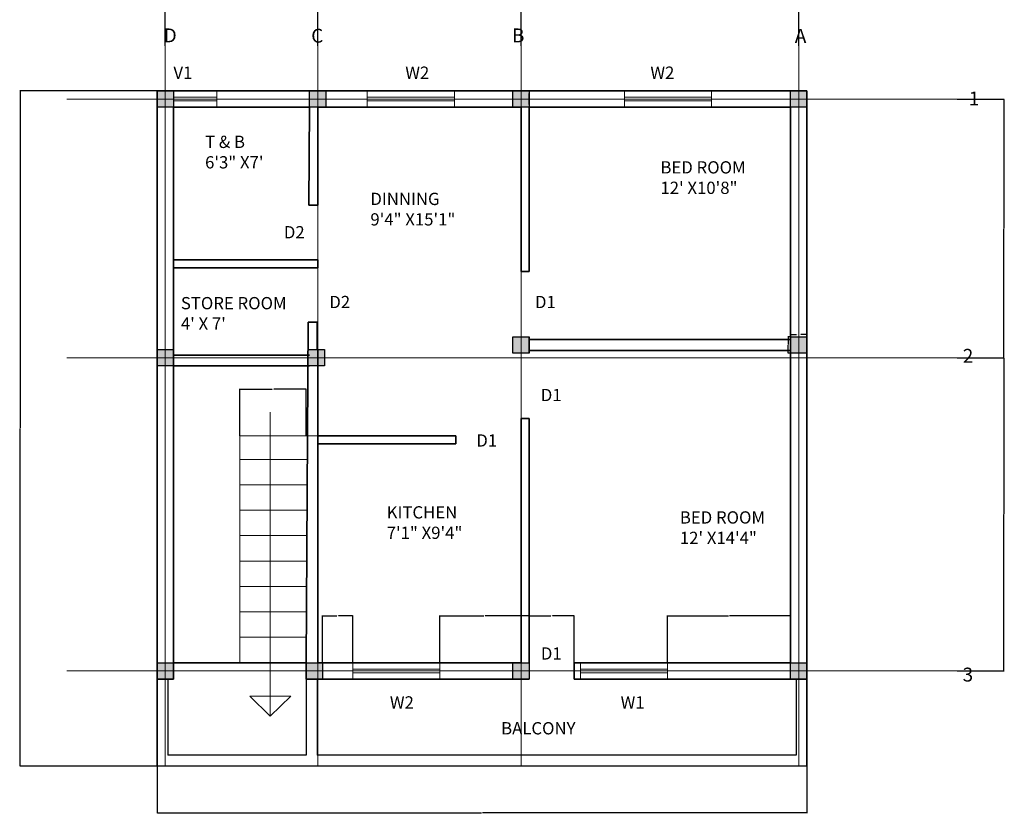
# Model space of a CAD drawing. Units: inches. Extents: x 3504 to 4623, y 2365 to 3357.
# Tile 4 of 5: x 4081 to 4623, y 2365 to 2803. Entities that reach past the tile are written whole.
import ezdxf

# ---------------------------------------------------------------- set-up
doc = ezdxf.new("R2010")
doc.units = ezdxf.units.IN
for name, color, linetype, lineweight in [('A-ANNO-DIMS', 2, 'Continuous', 18), ('A-ANNO-SYMB', 150, 'Continuous', 18), ('A-ANNO-TEXT', 7, 'Continuous', 18), ('A-AREA-IDEN', 7, 'Continuous', 18), ('A-FLOR-HRAL', 7, 'Continuous', 25), ('A-FLOR-STRS', 7, 'Continuous', 18), ('A-GLAZ', 4, 'Continuous', 18), ('A-GRID', 150, 'Continuous', 13), ('A-GRID-IDEN', 7, 'Continuous', 18), ('A-WALL', 7, 'Continuous', 35)]:
    doc.layers.add(name, color=color, linetype=linetype, lineweight=lineweight)
doc.layers.add('S-COLS', color=244, linetype='Continuous', lineweight=30, true_color=0x991b1e)
doc.layers.add('S-COLS-PATT', color=244, linetype='Continuous', lineweight=13, true_color=0x991b1e)
doc.styles.get("Standard").update_dxf_attribs({"font": 'arial.ttf'})
doc.dimstyles.get("Standard").update_dxf_attribs({"dimtxt": 0.18, "dimasz": 0.18, "dimexe": 0.18, "dimexo": 0.0625, "dimgap": 0.09, "dimtad": 0, "dimtih": 1, "dimtoh": 1, "dimdec": 4, "dimzin": 0, "dimdsep": 46, "dimtxsty": 'Standard', "dimcen": 0.09, "dimadec": 0, "dimazin": 0, "dimtfac": 1, "dimtdec": 4, "dimtofl": 0, "dimtmove": 0, "dimatfit": 3, "dimfxl": 1, "dimtolj": 1, "dimtzin": 0, "dimarcsym": 0})

# ---------------------------------------------------------------- blocks, each defined once
blk = doc.blocks.new('WIN-48-PLAN')
for p, q in [((48, 5.5), (0, 5.5)), ((48, 3.5), (0, 3.5)), ((48, 3.5), (0, 3.5))]:
    blk.add_line(p, q)
blk.add_lwpolyline([(48, 9), (48, 0), (0, 0), (0, 9)], close=True)
blk = doc.blocks.new('VENT-24-PLAN')
for p, q in [((0, 0), (0, 9)), ((0, 9), (24, 9)), ((24, 5.5), (0, 5.5)), ((24, 9), (24, 0)), ((24, 3.5), (0, 3.5)), ((24, 3.5), (0, 3.5)), ((24, 0), (0, 0))]:
    blk.add_line(p, q)
blk = doc.blocks.new('COL-9-SQUARE')
h = blk.add_hatch(color=256)
h.dxf.hatch_style = 1
h.paths.add_polyline_path([(9, 9), (0, 9), (0, 0), (9, 0)])
blk.add_lwpolyline([(0, 9), (9, 9), (9, 0), (0, 0)], close=True)
blk = doc.blocks.new('COL-9-PERIMETER')
h = blk.add_hatch(color=256)
h.dxf.hatch_style = 1
h.paths.add_polyline_path([(9, 9), (0, 9), (0, 0), (9, 0)])
for p, q in [((0, 9), (9, 9)), ((0, 0), (0, 9)), ((9, 9), (9, 0)), ((9, 0), (0, 0))]:
    blk.add_line(p, q)
blk = doc.blocks.new('COL-9-PARTITION-HEAD')
h = blk.add_hatch(color=256)
h.dxf.hatch_style = 1
h.paths.add_polyline_path([(9, 9), (0, 9), (0, 4.5), (0, 0), (9, 0)])
blk.add_line((9, 1.5), (9, 7.5))
blk.add_lwpolyline([(0, 9), (9, 9), (9, 0), (0, 0), (0, 4.5)], close=True)
blk = doc.blocks.new('*D13')
at = {"layer": 'A-ANNO-DIMS', "color": 0, "lineweight": -2, "transparency": 16777216}
for p, q in [((4505.45, 2627.94), (4505.45, 2629.41)), ((4505.63, 2629.23), (4508.78, 2629.23)), ((4514.27, 2629.23), (4511.12, 2629.23)), ((4514.45, 2627.94), (4514.45, 2629.41))]:
    blk.add_line(p, q, dxfattribs=at)
at = {"layer": 'A-ANNO-DIMS', "color": 0, "transparency": 16777216}
for points in [[(4505.63, 2629.26), (4505.63, 2629.2), (4505.45, 2629.23)], [(4514.27, 2629.26), (4514.27, 2629.2), (4514.45, 2629.23)]]:
    blk.add_solid(points, dxfattribs=at)
at = {"layer": 'Defpoints', "color": 0, "transparency": 16777216}
for p in [(4505.45, 2627.88), (4514.45, 2629.23), (4514.45, 2627.88)]:
    blk.add_point(p, dxfattribs=at)
at = {"layer": 'A-ANNO-DIMS', "color": 0, "transparency": 16777216, "insert": (4509.95, 2629.23), "char_height": 0.18, "attachment_point": 5}
blk.add_mtext('\\A1;EDGE COL. 9 TYP.', dxfattribs=at)
blk = doc.blocks.new('*D14')
at = {"layer": 'A-ANNO-DIMS', "color": 0, "lineweight": -2, "transparency": 16777216}
for p, q in [((4505.39, 2627.88), (4503.92, 2627.88)), ((4504.1, 2627.7), (4504.1, 2623.56)), ((4504.1, 2619.06), (4504.1, 2623.2)), ((4505.39, 2618.88), (4503.92, 2618.88))]:
    blk.add_line(p, q, dxfattribs=at)
at = {"layer": 'A-ANNO-DIMS', "color": 0, "transparency": 16777216}
for points in [[(4504.07, 2627.7), (4504.13, 2627.7), (4504.1, 2627.88)], [(4504.07, 2619.06), (4504.13, 2619.06), (4504.1, 2618.88)]]:
    blk.add_solid(points, dxfattribs=at)
at = {"layer": 'Defpoints', "color": 0, "transparency": 16777216}
for p in [(4504.1, 2627.88), (4505.45, 2627.88), (4505.45, 2618.88)]:
    blk.add_point(p, dxfattribs=at)
at = {"layer": 'A-ANNO-DIMS', "color": 0, "transparency": 16777216, "insert": (4504.1, 2623.38), "char_height": 0.18, "attachment_point": 5}
blk.add_mtext('\\A1;9 TYP.', dxfattribs=at)
blk = doc.blocks.new('*D35')
at = {"layer": 'A-ANNO-DIMS', "color": 0, "lineweight": -2, "transparency": 16777216}
for p, q in [((4156.45, 2391.3), (4156.45, 2365.43)), ((4514.45, 2391.3), (4514.45, 2365.43)), ((4156.63, 2365.61), (4335.16, 2365.61)), ((4514.27, 2365.61), (4335.74, 2365.61))]:
    blk.add_line(p, q, dxfattribs=at)
at = {"layer": 'A-ANNO-DIMS', "color": 0, "transparency": 16777216}
for points in [[(4156.63, 2365.64), (4156.63, 2365.58), (4156.45, 2365.61)], [(4514.27, 2365.64), (4514.27, 2365.58), (4514.45, 2365.61)]]:
    blk.add_solid(points, dxfattribs=at)
at = {"layer": 'Defpoints', "color": 0, "transparency": 16777216}
for p in [(4156.45, 2391.36), (4514.45, 2391.36), (4514.45, 2365.61)]:
    blk.add_point(p, dxfattribs=at)
at = {"layer": 'A-ANNO-DIMS', "color": 0, "transparency": 16777216, "insert": (4335.45, 2365.61), "char_height": 0.18, "attachment_point": 5}
blk.add_mtext('\\A1;358', dxfattribs=at)
blk = doc.blocks.new('*D36')
at = {"layer": 'A-ANNO-DIMS', "color": 0, "lineweight": -2, "transparency": 16777216}
for p, q in [((4156.39, 2763.36), (4080.79, 2763.36)), ((4080.97, 2763.18), (4080.97, 2577.54)), ((4080.97, 2391.54), (4080.97, 2577.18)), ((4156.39, 2391.36), (4080.79, 2391.36))]:
    blk.add_line(p, q, dxfattribs=at)
at = {"layer": 'A-ANNO-DIMS', "color": 0, "transparency": 16777216}
for points in [[(4080.94, 2763.18), (4081, 2763.18), (4080.97, 2763.36)], [(4080.94, 2391.54), (4081, 2391.54), (4080.97, 2391.36)]]:
    blk.add_solid(points, dxfattribs=at)
at = {"layer": 'Defpoints', "color": 0, "transparency": 16777216}
for p in [(4080.97, 2763.36), (4156.45, 2763.36), (4156.45, 2391.36)]:
    blk.add_point(p, dxfattribs=at)
at = {"layer": 'A-ANNO-DIMS', "color": 0, "transparency": 16777216, "insert": (4080.97, 2577.36), "char_height": 0.18, "attachment_point": 5}
blk.add_mtext('\\A1;372', dxfattribs=at)
blk = doc.blocks.new('*D37')
at = {"layer": 'A-ANNO-DIMS', "color": 0, "lineweight": -2, "transparency": 16777216}
for p, q in [((4160.95, 2788.12), (4160.95, 2813.99)), ((4161.13, 2813.81), (4202.73, 2813.81)), ((4244.77, 2813.81), (4203.17, 2813.81)), ((4244.95, 2788.12), (4244.95, 2813.99))]:
    blk.add_line(p, q, dxfattribs=at)
at = {"layer": 'A-ANNO-DIMS', "color": 0, "transparency": 16777216}
for points in [[(4161.13, 2813.84), (4161.13, 2813.78), (4160.95, 2813.81)], [(4244.77, 2813.84), (4244.77, 2813.78), (4244.95, 2813.81)]]:
    blk.add_solid(points, dxfattribs=at)
at = {"layer": 'Defpoints', "color": 0, "transparency": 16777216}
for p in [(4244.95, 2813.81), (4160.95, 2788.06), (4244.95, 2788.06)]:
    blk.add_point(p, dxfattribs=at)
at = {"layer": 'A-ANNO-DIMS', "color": 0, "transparency": 16777216, "insert": (4202.95, 2813.81), "char_height": 0.18, "attachment_point": 5}
blk.add_mtext('\\A1;84', dxfattribs=at)
blk = doc.blocks.new('*D38')
at = {"layer": 'A-ANNO-DIMS', "color": 0, "lineweight": -2, "transparency": 16777216}
for p, q in [((4244.95, 2788.12), (4244.95, 2813.99)), ((4245.13, 2813.81), (4300.67, 2813.81)), ((4356.77, 2813.81), (4301.23, 2813.81)), ((4356.95, 2788.12), (4356.95, 2813.99))]:
    blk.add_line(p, q, dxfattribs=at)
at = {"layer": 'A-ANNO-DIMS', "color": 0, "transparency": 16777216}
for points in [[(4245.13, 2813.84), (4245.13, 2813.78), (4244.95, 2813.81)], [(4356.77, 2813.84), (4356.77, 2813.78), (4356.95, 2813.81)]]:
    blk.add_solid(points, dxfattribs=at)
at = {"layer": 'Defpoints', "color": 0, "transparency": 16777216}
for p in [(4356.95, 2813.81), (4244.95, 2788.06), (4356.95, 2788.06)]:
    blk.add_point(p, dxfattribs=at)
at = {"layer": 'A-ANNO-DIMS', "color": 0, "transparency": 16777216, "insert": (4300.95, 2813.81), "char_height": 0.18, "attachment_point": 5}
blk.add_mtext('\\A1;112', dxfattribs=at)
blk = doc.blocks.new('*D39')
at = {"layer": 'A-ANNO-DIMS', "color": 0, "lineweight": -2, "transparency": 16777216}
for p, q in [((4356.95, 2788.12), (4356.95, 2813.99)), ((4357.13, 2813.81), (4433.17, 2813.81)), ((4509.77, 2813.81), (4433.73, 2813.81)), ((4509.95, 2788.12), (4509.95, 2813.99))]:
    blk.add_line(p, q, dxfattribs=at)
at = {"layer": 'A-ANNO-DIMS', "color": 0, "transparency": 16777216}
for points in [[(4357.13, 2813.84), (4357.13, 2813.78), (4356.95, 2813.81)], [(4509.77, 2813.84), (4509.77, 2813.78), (4509.95, 2813.81)]]:
    blk.add_solid(points, dxfattribs=at)
at = {"layer": 'Defpoints', "color": 0, "transparency": 16777216}
for p in [(4509.95, 2813.81), (4356.95, 2788.06), (4509.95, 2788.06)]:
    blk.add_point(p, dxfattribs=at)
at = {"layer": 'A-ANNO-DIMS', "color": 0, "transparency": 16777216, "insert": (4433.45, 2813.81), "char_height": 0.18, "attachment_point": 5}
blk.add_mtext('\\A1;153', dxfattribs=at)
blk = doc.blocks.new('*D40')
at = {"layer": 'A-ANNO-DIMS', "color": 0, "lineweight": -2, "transparency": 16777216}
for p, q in [((4597.21, 2616.36), (4623.08, 2616.36)), ((4622.9, 2616.18), (4622.9, 2530.29)), ((4622.9, 2444.04), (4622.9, 2529.93)), ((4597.21, 2443.86), (4623.08, 2443.86))]:
    blk.add_line(p, q, dxfattribs=at)
at = {"layer": 'A-ANNO-DIMS', "color": 0, "transparency": 16777216}
for points in [[(4622.87, 2616.18), (4622.93, 2616.18), (4622.9, 2616.36)], [(4622.87, 2444.04), (4622.93, 2444.04), (4622.9, 2443.86)]]:
    blk.add_solid(points, dxfattribs=at)
at = {"layer": 'Defpoints', "color": 0, "transparency": 16777216}
for p in [(4597.15, 2616.36), (4622.9, 2616.36), (4597.15, 2443.86)]:
    blk.add_point(p, dxfattribs=at)
at = {"layer": 'A-ANNO-DIMS', "color": 0, "transparency": 16777216, "insert": (4622.9, 2530.11), "char_height": 0.18, "attachment_point": 5}
blk.add_mtext('\\A1;172.5', dxfattribs=at)
blk = doc.blocks.new('*D41')
at = {"layer": 'A-ANNO-DIMS', "color": 0, "lineweight": -2, "transparency": 16777216}
for p, q in [((4597.21, 2758.86), (4623.08, 2758.86)), ((4622.9, 2758.68), (4622.9, 2687.79)), ((4622.9, 2616.54), (4622.9, 2687.43)), ((4597.21, 2616.36), (4623.08, 2616.36))]:
    blk.add_line(p, q, dxfattribs=at)
at = {"layer": 'A-ANNO-DIMS', "color": 0, "transparency": 16777216}
for points in [[(4622.87, 2758.68), (4622.93, 2758.68), (4622.9, 2758.86)], [(4622.87, 2616.54), (4622.93, 2616.54), (4622.9, 2616.36)]]:
    blk.add_solid(points, dxfattribs=at)
at = {"layer": 'Defpoints', "color": 0, "transparency": 16777216}
for p in [(4597.15, 2758.86), (4622.9, 2758.86), (4597.15, 2616.36)]:
    blk.add_point(p, dxfattribs=at)
at = {"layer": 'A-ANNO-DIMS', "color": 0, "transparency": 16777216, "insert": (4622.9, 2687.61), "char_height": 0.18, "attachment_point": 5}
blk.add_mtext('\\A1;142.5', dxfattribs=at)
blk = doc.blocks.new('*D42')
at = {"layer": 'A-ANNO-DIMS', "color": 0, "lineweight": -2, "transparency": 16777216}
for p, q in [((4247.62, 2448.42), (4247.62, 2474.29)), ((4247.8, 2474.11), (4255.56, 2474.11)), ((4264.08, 2474.11), (4256.33, 2474.11)), ((4264.26, 2448.42), (4264.26, 2474.29))]:
    blk.add_line(p, q, dxfattribs=at)
at = {"layer": 'A-ANNO-DIMS', "color": 0, "transparency": 16777216}
for points in [[(4247.8, 2474.14), (4247.8, 2474.08), (4247.62, 2474.11)], [(4264.08, 2474.14), (4264.08, 2474.08), (4264.26, 2474.11)]]:
    blk.add_solid(points, dxfattribs=at)
at = {"layer": 'Defpoints', "color": 0, "transparency": 16777216}
for p in [(4264.26, 2474.11), (4247.62, 2448.36), (4264.26, 2448.36)]:
    blk.add_point(p, dxfattribs=at)
at = {"layer": 'A-ANNO-DIMS', "color": 0, "transparency": 16777216, "insert": (4255.94, 2474.11), "char_height": 0.18, "attachment_point": 5}
blk.add_mtext('\\A1;16.64', dxfattribs=at)
blk = doc.blocks.new('*D43')
at = {"layer": 'A-ANNO-DIMS', "color": 0, "lineweight": -2, "transparency": 16777216}
for p, q in [((4312.26, 2448.42), (4312.26, 2474.29)), ((4312.44, 2474.11), (4336.46, 2474.11)), ((4361.27, 2474.11), (4337.25, 2474.11)), ((4361.45, 2448.42), (4361.45, 2474.29))]:
    blk.add_line(p, q, dxfattribs=at)
at = {"layer": 'A-ANNO-DIMS', "color": 0, "transparency": 16777216}
for points in [[(4312.44, 2474.14), (4312.44, 2474.08), (4312.26, 2474.11)], [(4361.27, 2474.14), (4361.27, 2474.08), (4361.45, 2474.11)]]:
    blk.add_solid(points, dxfattribs=at)
at = {"layer": 'Defpoints', "color": 0, "transparency": 16777216}
for p in [(4361.45, 2474.11), (4312.26, 2448.36), (4361.45, 2448.36)]:
    blk.add_point(p, dxfattribs=at)
at = {"layer": 'A-ANNO-DIMS', "color": 0, "transparency": 16777216, "insert": (4336.86, 2474.11), "char_height": 0.18, "attachment_point": 5}
blk.add_mtext('\\A1;49.19', dxfattribs=at)
blk = doc.blocks.new('*D44')
at = {"layer": 'A-ANNO-DIMS', "color": 0, "lineweight": -2, "transparency": 16777216}
for p, q in [((4361.45, 2448.42), (4361.45, 2474.29)), ((4361.63, 2474.11), (4373.39, 2474.11)), ((4386.09, 2474.11), (4374.32, 2474.11)), ((4386.27, 2448.42), (4386.27, 2474.29))]:
    blk.add_line(p, q, dxfattribs=at)
at = {"layer": 'A-ANNO-DIMS', "color": 0, "transparency": 16777216}
for points in [[(4361.63, 2474.14), (4361.63, 2474.08), (4361.45, 2474.11)], [(4386.09, 2474.14), (4386.09, 2474.08), (4386.27, 2474.11)]]:
    blk.add_solid(points, dxfattribs=at)
at = {"layer": 'Defpoints', "color": 0, "transparency": 16777216}
for p in [(4386.27, 2474.11), (4361.45, 2448.36), (4386.27, 2448.36)]:
    blk.add_point(p, dxfattribs=at)
at = {"layer": 'A-ANNO-DIMS', "color": 0, "transparency": 16777216, "insert": (4373.86, 2474.11), "char_height": 0.18, "attachment_point": 5}
blk.add_mtext('\\A1;24.817', dxfattribs=at)
blk = doc.blocks.new('*D45')
at = {"layer": 'A-ANNO-DIMS', "color": 0, "lineweight": -2, "transparency": 16777216}
for p, q in [((4437.65, 2448.42), (4437.65, 2474.29)), ((4437.83, 2474.11), (4471.23, 2474.11)), ((4505.27, 2474.11), (4471.87, 2474.11)), ((4505.45, 2448.42), (4505.45, 2474.29))]:
    blk.add_line(p, q, dxfattribs=at)
at = {"layer": 'A-ANNO-DIMS', "color": 0, "transparency": 16777216}
for points in [[(4437.83, 2474.14), (4437.83, 2474.08), (4437.65, 2474.11)], [(4505.27, 2474.14), (4505.27, 2474.08), (4505.45, 2474.11)]]:
    blk.add_solid(points, dxfattribs=at)
at = {"layer": 'Defpoints', "color": 0, "transparency": 16777216}
for p in [(4505.45, 2474.11), (4437.65, 2448.36), (4505.45, 2448.36)]:
    blk.add_point(p, dxfattribs=at)
at = {"layer": 'A-ANNO-DIMS', "color": 0, "transparency": 16777216, "insert": (4471.55, 2474.11), "char_height": 0.18, "attachment_point": 5}
blk.add_mtext('\\A1;67.8', dxfattribs=at)
blk = doc.blocks.new('*D46')
at = {"layer": 'A-ANNO-DIMS', "color": 0, "lineweight": -2, "transparency": 16777216}
for p, q in [((4202.04, 2573.42), (4202.04, 2599.29)), ((4202.22, 2599.11), (4219.86, 2599.11)), ((4238.44, 2599.11), (4220.79, 2599.11)), ((4238.62, 2573.42), (4238.62, 2599.29))]:
    blk.add_line(p, q, dxfattribs=at)
at = {"layer": 'A-ANNO-DIMS', "color": 0, "transparency": 16777216}
for points in [[(4202.22, 2599.14), (4202.22, 2599.08), (4202.04, 2599.11)], [(4238.44, 2599.14), (4238.44, 2599.08), (4238.62, 2599.11)]]:
    blk.add_solid(points, dxfattribs=at)
at = {"layer": 'Defpoints', "color": 0, "transparency": 16777216}
for p in [(4238.62, 2599.11), (4202.04, 2573.36), (4238.62, 2573.36)]:
    blk.add_point(p, dxfattribs=at)
at = {"layer": 'A-ANNO-DIMS', "color": 0, "transparency": 16777216, "insert": (4220.33, 2599.11), "char_height": 0.18, "attachment_point": 5}
blk.add_mtext('\\A1;36.585', dxfattribs=at)

msp = doc.modelspace()

# ---------------------------------------------------------------- hatches: boundary and pattern name
at = {"layer": 'S-COLS-PATT'}
h = msp.add_hatch(color=256, dxfattribs=at)
h.dxf.hatch_style = 1
h.paths.add_polyline_path([(4361.4512, 2627.8606), (4352.4512, 2627.8606), (4352.4512, 2623.3606), (4352.4512, 2618.8606), (4361.4512, 2618.8606)])
h.paths.add_polyline_path([(4361.4512, 2448.3606), (4352.4512, 2448.3606), (4352.4512, 2443.8606), (4352.4512, 2439.3606), (4361.4512, 2439.3606)])

# ---------------------------------------------------------------- linework, layer by layer
at = {"layer": 'A-ANNO-SYMB'}
for p, q in [((4218.6823, 2586.3138), (4218.6823, 2418.8848)), ((4218.6823, 2418.8848), (4207.6157, 2429.9514)), ((4207.6157, 2429.9514), (4230.1811, 2429.9514)), ((4230.1811, 2429.9514), (4218.6823, 2418.8848))]:
    msp.add_line(p, q, dxfattribs=at)
at = {"layer": 'A-FLOR-HRAL'}
for p, q in [((4156.4512, 2439.3606), (4156.4512, 2391.3606)), ((4162.4512, 2439.3606), (4162.4512, 2397.3606)), ((4238.6215, 2439.3606), (4238.6215, 2397.3606)), ((4244.6215, 2439.3606), (4244.6215, 2397.3606)), ((4508.4512, 2439.3606), (4508.4512, 2397.3606)), ((4514.4512, 2439.3606), (4514.4512, 2391.3606)), ((4238.6215, 2397.3606), (4162.4512, 2397.3606)), ((4361.4512, 2397.3606), (4244.6215, 2397.3606)), ((4508.4512, 2397.3606), (4361.4512, 2397.3606)), ((4361.4512, 2391.3606), (4156.4512, 2391.3606)), ((4514.4512, 2391.3606), (4361.4512, 2391.3606))]:
    msp.add_line(p, q, dxfattribs=at)
at = {"layer": 'A-FLOR-STRS'}
for p, q in [((4244.9512, 2573.3606), (4202.0364, 2573.3606)), ((4202.0364, 2573.3606), (4238.6215, 2573.3606)), ((4202.0364, 2448.3606), (4202.0364, 2573.3606)), ((4202.0364, 2560.3586), (4239.2912, 2560.3586)), ((4202.0364, 2546.3588), (4239.2075, 2546.3588)), ((4202.0364, 2532.3591), (4239.1238, 2532.3591)), ((4202.0364, 2518.3593), (4239.0401, 2518.3593)), ((4202.0364, 2504.3596), (4238.9563, 2504.3596)), ((4202.0364, 2490.3598), (4238.8726, 2490.3598)), ((4202.0364, 2476.3601), (4238.7889, 2476.3601)), ((4202.0364, 2462.3603), (4238.7052, 2462.3603))]:
    msp.add_line(p, q, dxfattribs=at)
at = {"layer": 'A-GRID'}
for p, q in [((4160.9512, 2788.0584), (4160.9512, 2391.3606)), ((4244.9512, 2788.0584), (4244.9512, 2391.3606)), ((4356.9512, 2788.0584), (4356.9512, 2391.3606)), ((4509.9512, 2788.0584), (4509.9512, 2391.3606)), ((4106.7158, 2758.8606), (4597.1464, 2758.8606)), ((4106.7158, 2616.3606), (4597.1464, 2616.3606)), ((4106.7158, 2443.8606), (4361.4512, 2443.8606)), ((4352.4512, 2443.8606), (4597.1464, 2443.8606))]:
    msp.add_line(p, q, dxfattribs=at)
at = {"layer": 'A-WALL'}
for p, q in [((4156.4512, 2439.3606), (4156.4512, 2763.3606)), ((4514.4512, 2763.3606), (4156.4512, 2763.3606)), ((4156.4512, 2763.3606), (4156.4512, 2391.3606)), ((4514.4512, 2439.3606), (4514.4512, 2763.3606)), ((4514.4512, 2763.3606), (4514.4512, 2391.3606)), ((4165.4512, 2474.3606), (4165.4512, 2754.3606)), ((4240.4512, 2754.3606), (4165.4512, 2754.3606)), ((4240.1285, 2700.3894), (4240.4512, 2754.3606)), ((4244.9512, 2700.3606), (4244.9512, 2754.3606)), ((4356.9512, 2754.3606), (4244.9512, 2754.3606)), ((4356.9512, 2663.8606), (4356.9512, 2754.3606)), ((4361.4512, 2663.8606), (4361.4512, 2754.3606)), ((4505.4512, 2754.3606), (4361.4512, 2754.3606)), ((4505.4512, 2448.3606), (4505.4512, 2754.3606)), ((4244.9512, 2700.3606), (4240.1285, 2700.3894)), ((4240.4512, 2670.3606), (4165.4512, 2670.3606)), ((4239.949, 2670.3606), (4244.9512, 2670.3606)), ((4244.9512, 2665.8606), (4244.9512, 2670.3606)), ((4239.9221, 2665.8606), (4165.4512, 2665.8606)), ((4239.9221, 2665.8606), (4244.9512, 2665.8606)), ((4356.9512, 2663.8606), (4361.4512, 2663.8606)), ((4238.6215, 2448.3606), (4239.7428, 2635.8912)), ((4244.736, 2635.8614), (4239.7428, 2635.8912)), ((4244.736, 2635.8614), (4244.736, 2620.8606)), ((4505.4512, 2626.3606), (4361.4512, 2626.3606)), ((4244.9512, 2448.3606), (4244.9512, 2620.8606)), ((4505.4512, 2620.3606), (4361.4512, 2620.3606)), ((4240.4512, 2617.8606), (4165.4512, 2617.8606)), ((4240.4512, 2611.8606), (4165.4512, 2611.8606)), ((4356.9512, 2448.3606), (4356.9512, 2582.8606)), ((4356.9512, 2582.8606), (4361.4512, 2582.8606)), ((4361.4512, 2448.3606), (4361.4512, 2582.8606)), ((4320.9512, 2573.3606), (4244.9512, 2573.3606)), ((4320.9512, 2573.3606), (4320.9512, 2568.8606)), ((4320.9512, 2568.8606), (4244.9512, 2568.8606)), ((4165.4512, 2448.3606), (4165.4512, 2474.3606)), ((4165.4512, 2448.3606), (4238.6215, 2448.3606)), ((4165.4512, 2448.3606), (4165.4512, 2439.3606)), ((4238.6215, 2448.3606), (4238.6215, 2439.3606)), ((4356.9512, 2448.3606), (4244.9512, 2448.3606)), ((4505.4512, 2448.3606), (4386.2684, 2448.3606)), ((4386.2684, 2448.3606), (4386.2684, 2439.3606)), ((4162.4512, 2439.3606), (4156.4512, 2439.3606)), ((4165.4512, 2439.3606), (4162.4512, 2439.3606)), ((4361.4512, 2439.3606), (4238.6215, 2439.3606)), ((4514.4512, 2439.3606), (4386.2684, 2439.3606))]:
    msp.add_line(p, q, dxfattribs=at)
at = {"layer": 'S-COLS'}
for p, q in [((4361.4512, 2626.3606), (4361.4512, 2627.8606)), ((4361.4512, 2620.3606), (4361.4512, 2626.3606)), ((4361.4512, 2618.8606), (4361.4512, 2620.3606))]:
    msp.add_line(p, q, dxfattribs=at)
for points in [[(4352.4512, 2627.8606), (4361.4512, 2627.8606), (4361.4512, 2618.8606), (4352.4512, 2618.8606), (4352.4512, 2623.3606)], [(4352.4512, 2448.3606), (4361.4512, 2448.3606), (4361.4512, 2439.3606), (4352.4512, 2439.3606), (4352.4512, 2443.8606)]]:
    msp.add_lwpolyline(points, close=True, dxfattribs=at)

# ---------------------------------------------------------------- block references
at = {"layer": 'A-GLAZ'}
for name, p in [('VENT-24-PLAN', (4165.4512, 2754.3606)), ('WIN-48-PLAN', (4272.221, 2754.3606)), ('WIN-48-PLAN', (4413.9621, 2754.3606)), ('WIN-48-PLAN', (4264.2605, 2439.3606)), ('WIN-48-PLAN', (4389.6491, 2439.3606))]:
    msp.add_blockref(name, p, dxfattribs=at)
at = {"layer": 'S-COLS'}
for name, p in [('COL-9-SQUARE', (4156.4512, 2754.3606)), ('COL-9-SQUARE', (4240.4512, 2754.3606)), ('COL-9-PARTITION-HEAD', (4352.4512, 2754.3606)), ('COL-9-PERIMETER', (4505.4512, 2754.3606)), ('COL-9-PERIMETER', (4505.4512, 2618.8797)), ('COL-9-SQUARE', (4156.4512, 2611.8606)), ('COL-9-SQUARE', (4239.5992, 2611.8606)), ('COL-9-SQUARE', (4156.4512, 2439.3606)), ('COL-9-SQUARE', (4238.6215, 2439.3606)), ('COL-9-PERIMETER', (4505.4512, 2439.3606))]:
    msp.add_blockref(name, p, dxfattribs=at)

# ---------------------------------------------------------------- texts
at = {"layer": 'A-ANNO-TEXT', "char_height": 6.7599, "attachment_point": 1}
for s, insert in [('V1', (4165.4512, 2776.7302)), ('W2', (4293.1898, 2776.7302)), ('W2', (4428.213, 2776.7302)), ('D2', (4226.2985, 2688.8505)), ('D2', (4251.3465, 2650.4275)), ('D1', (4364.6452, 2650.4275)), ('D1', (4367.849, 2599.197)), ('D1', (4332.3157, 2574.1639)), ('D1', (4367.8799, 2456.8443)), ('W2', (4284.7021, 2429.8749)), ('W1', (4411.8276, 2429.8749))]:
    msp.add_mtext_dynamic_manual_height_columns(s, width=979.683598, gutter_width=33.7995, heights=[43.6273], dxfattribs=dict(at, insert=insert))
at = {"layer": 'A-AREA-IDEN', "attachment_point": 1}
for s, insert, char_height in [('T & B \\P6\'3" X7\'', (4182.894, 2738.6463), 6.7599), ('BED ROOM \\P12\' X10\'8"', (4433.7699, 2724.5921), 6.7599), ('DINNING\\P9\'4" X15\'1"', (4273.9619, 2707.2184), 6.759897), ("STORE ROOM \\P4' X 7'", (4169.5579, 2649.793), 6.759897), ('KITCHEN\\P7\'1" X9\'4"', (4282.9512, 2534.5796), 6.7599), ('BED ROOM\\P12\' X14\'4"', (4444.4574, 2531.7688), 6.7599), ('BALCONY', (4345.9985, 2415.6452), 6.7599)]:
    msp.add_mtext_dynamic_manual_height_columns(s, width=979.683598, gutter_width=33.7995, heights=[43.6273], dxfattribs=dict(at, insert=insert, char_height=char_height))
at = {"layer": 'A-GRID-IDEN', "attachment_point": 1}
for s, insert, char_height in [('D ', (4160.1004, 2797.7111), 7.62721), ('C ', (4241.3664, 2797.5368), 7.62721), ('B ', (4351.9944, 2797.7111), 7.62721), ('A ', (4507.7848, 2797.4127), 7.62721), ('1', (4603.6204, 2762.9672), 7.6272), ('2 ', (4600.3399, 2621.2138), 7.62721), ('3 ', (4600.2519, 2445.656), 7.62721)]:
    msp.add_mtext_dynamic_manual_height_columns(s, width=55.225033, gutter_width=38.1361, heights=[0], dxfattribs=dict(at, insert=insert, char_height=char_height))

# ---------------------------------------------------------------- dimensions: what is measured, and where the dimension line sits
at = {"layer": 'A-ANNO-DIMS'}
for base, p1, p2, override, picture, middle in [((4244.9512, 2813.8084), (4160.9512, 2788.0584), (4244.9512, 2788.0584), {"dimdec": 0, "dimlfac": 1, "dimrnd": 0, "dimzin": 0, "dimdsep": 46, "dimlunit": 2}, '*D37', (4202.9512, 2813.8084)), ((4356.9512, 2813.8084), (4244.9512, 2788.0584), (4356.9512, 2788.0584), {"dimdec": 0, "dimlfac": 1, "dimrnd": 0, "dimzin": 0, "dimdsep": 46, "dimlunit": 2}, '*D38', (4300.9512, 2813.8084)), ((4509.9512, 2813.8084), (4356.9512, 2788.0584), (4509.9512, 2788.0584), {"dimdec": 0, "dimlfac": 1, "dimrnd": 0, "dimzin": 0, "dimdsep": 46, "dimlunit": 2}, '*D39', (4433.4512, 2813.8084)), ((4264.2605, 2474.1106), (4247.6215, 2448.3606), (4264.2605, 2448.3606), {"dimdec": 2, "dimlfac": 1, "dimrnd": 0, "dimzin": 0, "dimdsep": 46, "dimlunit": 2}, '*D42', (4255.941, 2474.1106)), ((4361.4512, 2474.1106), (4312.2605, 2448.3606), (4361.4512, 2448.3606), {"dimdec": 2, "dimlfac": 1, "dimrnd": 0, "dimzin": 0, "dimdsep": 46, "dimlunit": 2}, '*D43', (4336.8559, 2474.1106)), ((4386.2684, 2474.1106), (4361.4512, 2448.3606), (4386.2684, 2448.3606), {"dimdec": 3, "dimlfac": 1, "dimrnd": 0, "dimzin": 0, "dimdsep": 46, "dimlunit": 2}, '*D44', (4373.8598, 2474.1106)), ((4505.4512, 2474.1106), (4437.6491, 2448.3606), (4505.4512, 2448.3606), {"dimdec": 1, "dimlfac": 1, "dimrnd": 0, "dimzin": 0, "dimdsep": 46, "dimlunit": 2}, '*D45', (4471.5502, 2474.1106)), ((4514.4512, 2365.6106), (4156.4512, 2391.3606), (4514.4512, 2391.3606), {"dimdec": 0, "dimlfac": 1, "dimrnd": 0, "dimzin": 0, "dimdsep": 46, "dimlunit": 2}, '*D35', (4335.4512, 2365.6106))]:
    dim = msp.add_linear_dim(base=base, p1=p1, p2=p2, dimstyle='Standard', override=override, dxfattribs=at)
    dim.commit()
    dim.dimension.update_dxf_attribs({"geometry": picture, "text_midpoint": middle})
for base, p1, p2, angle, override, picture, middle in [((4080.9658, 2763.3606), (4156.4512, 2391.3606), (4156.4512, 2763.3606), 90, {"dimdec": 0, "dimlfac": 1, "dimrnd": 0, "dimzin": 0, "dimdsep": 46, "dimlunit": 2}, '*D36', (4080.9658, 2577.3606)), ((4622.8964, 2758.8606), (4597.1464, 2616.3606), (4597.1464, 2758.8606), 90, {"dimdec": 1, "dimlfac": 1, "dimrnd": 0, "dimzin": 0, "dimdsep": 46, "dimlunit": 2}, '*D41', (4622.8964, 2687.6106)), ((4622.8964, 2616.3606), (4597.1464, 2443.8606), (4597.1464, 2616.3606), 90, {"dimdec": 1, "dimlfac": 1, "dimrnd": 0, "dimzin": 0, "dimdsep": 46, "dimlunit": 2}, '*D40', (4622.8964, 2530.1106)), ((4238.6215, 2599.1106), (4202.0364, 2573.3606), (4238.6215, 2573.3606), 0, {"dimdec": 3, "dimlfac": 1, "dimrnd": 0, "dimzin": 0, "dimdsep": 46, "dimlunit": 2}, '*D46', (4220.3289, 2599.1106))]:
    dim = msp.add_linear_dim(base=base, p1=p1, p2=p2, angle=angle, dimstyle='Standard', override=override, dxfattribs=at)
    dim.commit()
    dim.dimension.update_dxf_attribs({"geometry": picture, "text_midpoint": middle})
dim = msp.add_linear_dim(base=(4504.1012, 2627.8797), p1=(4505.4512, 2618.8797), p2=(4505.4512, 2627.8797), angle=90, text='<> TYP.', dimstyle='Standard', override={"dimdec": 0, "dimlfac": 1, "dimrnd": 0, "dimzin": 0, "dimdsep": 46, "dimlunit": 2}, dxfattribs=at)
dim.commit()
dim.dimension.update_dxf_attribs({"geometry": '*D14', "text_midpoint": (4504.1012, 2623.3797)})
dim = msp.add_linear_dim(base=(4514.4512, 2629.2297), p1=(4505.4512, 2627.8797), p2=(4514.4512, 2627.8797), text='EDGE COL. <> TYP.', dimstyle='Standard', override={"dimdec": 0, "dimlfac": 1, "dimrnd": 0, "dimzin": 0, "dimdsep": 46, "dimlunit": 2}, dxfattribs=at)
dim.commit()
dim.dimension.update_dxf_attribs({"geometry": '*D13', "text_midpoint": (4509.9512, 2629.2297)})

doc.saveas('drawing.dxf')
